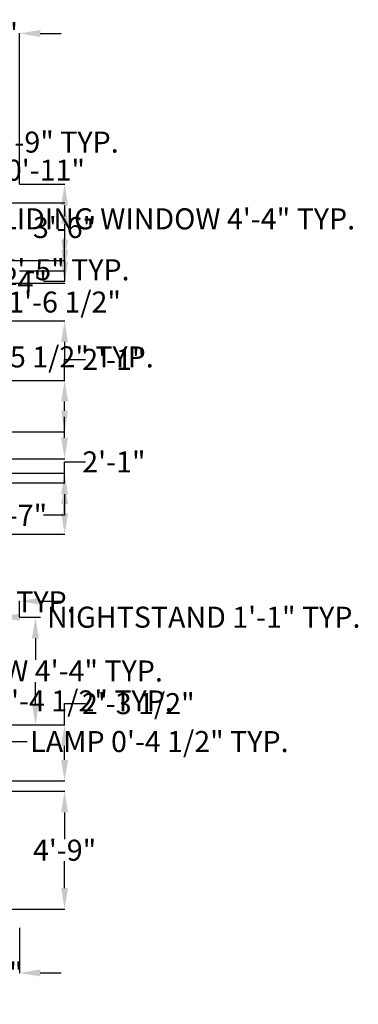
# Model space of a CAD drawing. Units: inches. Extents: x 19 to 1371, y 7 to 588.
# Tile 5 of 5: x 1207 to 1371, y 103 to 580. Entities that reach past the tile are written whole.
import ezdxf

# ---------------------------------------------------------------- set-up
doc = ezdxf.new("R2010")
doc.units = ezdxf.units.IN
doc.header["$MEASUREMENT"] = 0
doc.layers.add('A-ANNO-DIMS', color=2, linetype='Continuous', lineweight=18)
doc.styles.get("Standard").update_dxf_attribs({"font": 'arial.ttf'})
doc.dimstyles.get("Standard").update_dxf_attribs({"dimtxt": 10.18, "dimasz": 10.18, "dimexe": 0.18, "dimexo": 0.0625, "dimgap": 0.09, "dimtad": 0, "dimtih": 1, "dimtoh": 1, "dimdec": 0, "dimzin": 0, "dimdsep": 46, "dimlunit": 3, "dimtxsty": 'Standard', "dimcen": 0.09, "dimadec": 0, "dimazin": 0, "dimtfac": 1, "dimtdec": 0, "dimtofl": 0, "dimtmove": 0, "dimatfit": 3, "dimfxl": 1, "dimtolj": 1, "dimtzin": 0, "dimarcsym": 0})

# ---------------------------------------------------------------- blocks, each defined once
blk = doc.blocks.new('*D20')
at = {"layer": 'A-ANNO-DIMS', "color": 0, "lineweight": -2, "transparency": 16777216}
for p, q in [((1175.27, 490.89), (1185.12, 490.89)), ((1184.94, 480.71), (1184.94, 463.79)), ((1184.94, 436.16), (1184.94, 453.08)), ((1175.27, 425.98), (1185.12, 425.98))]:
    blk.add_line(p, q, dxfattribs=at)
at = {"layer": 'A-ANNO-DIMS', "color": 0, "transparency": 16777216}
for points in [[(1183.24, 480.71), (1186.64, 480.71), (1184.94, 490.89)], [(1183.24, 436.16), (1186.64, 436.16), (1184.94, 425.98)]]:
    blk.add_solid(points, dxfattribs=at)
at = {"layer": 'Defpoints', "color": 0, "transparency": 16777216}
for p in [(1175.2, 490.89), (1184.94, 490.89), (1175.2, 425.98)]:
    blk.add_point(p, dxfattribs=at)
at = {"layer": 'A-ANNO-DIMS', "color": 0, "transparency": 16777216, "insert": (1184.94, 458.44), "char_height": 10.18, "attachment_point": 5}
blk.add_mtext('\\A1;DOUBLE BED 5\'-5" TYP.', dxfattribs=at)
blk = doc.blocks.new('*D21')
at = {"layer": 'A-ANNO-DIMS', "color": 0, "lineweight": -2, "transparency": 16777216}
for p, q in [((1121.71, 425.92), (1121.71, 416.06)), ((1175.2, 425.92), (1175.2, 416.06)), ((1131.89, 416.24), (1165.02, 416.24)), ((1175.2, 416.24), (1185.38, 416.24))]:
    blk.add_line(p, q, dxfattribs=at)
at = {"layer": 'A-ANNO-DIMS', "color": 0, "transparency": 16777216}
for points in [[(1131.89, 417.94), (1131.89, 414.55), (1121.71, 416.24)], [(1165.02, 417.94), (1165.02, 414.55), (1175.2, 416.24)]]:
    blk.add_solid(points, dxfattribs=at)
at = {"layer": 'Defpoints', "color": 0, "transparency": 16777216}
for p in [(1121.71, 425.98), (1175.2, 425.98), (1175.2, 416.24)]:
    blk.add_point(p, dxfattribs=at)
at = {"layer": 'A-ANNO-DIMS', "color": 0, "transparency": 16777216, "insert": (1228.56, 416.24), "char_height": 10.18, "attachment_point": 5}
blk.add_mtext('\\A1;4\'-5 1/2" TYP.', dxfattribs=at)
blk = doc.blocks.new('*D22')
at = {"layer": 'A-ANNO-DIMS', "color": 0, "lineweight": -2, "transparency": 16777216}
for p, q in [((1183.48, 292.09), (1183.48, 290.03)), ((1196.42, 292.09), (1196.42, 290.03)), ((1173.3, 290.21), (1163.12, 290.21)), ((1206.6, 290.21), (1216.78, 290.21))]:
    blk.add_line(p, q, dxfattribs=at)
at = {"layer": 'A-ANNO-DIMS', "color": 0, "transparency": 16777216}
for points in [[(1173.3, 291.91), (1173.3, 288.52), (1183.48, 290.21)], [(1206.6, 291.91), (1206.6, 288.52), (1196.42, 290.21)]]:
    blk.add_solid(points, dxfattribs=at)
at = {"layer": 'Defpoints', "color": 0, "transparency": 16777216}
for p in [(1183.48, 292.15), (1196.42, 292.15), (1196.42, 290.21)]:
    blk.add_point(p, dxfattribs=at)
at = {"layer": 'A-ANNO-DIMS', "color": 0, "transparency": 16777216, "insert": (1295.84, 290.21), "char_height": 10.18, "attachment_point": 5}
blk.add_mtext('\\A1;NIGHTSTAND 1\'-1" TYP.', dxfattribs=at)
blk = doc.blocks.new('*D23')
at = {"layer": 'A-ANNO-DIMS', "color": 0, "lineweight": -2, "transparency": 16777216}
for p, q in [((1198.36, 313.34), (1198.36, 323.52)), ((1196.48, 303.16), (1198.54, 303.16)), ((1196.48, 292.15), (1198.54, 292.15)), ((1198.36, 281.97), (1198.36, 271.79))]:
    blk.add_line(p, q, dxfattribs=at)
at = {"layer": 'A-ANNO-DIMS', "color": 0, "transparency": 16777216}
for points in [[(1196.66, 313.34), (1200.05, 313.34), (1198.36, 303.16)], [(1196.66, 281.97), (1200.05, 281.97), (1198.36, 292.15)]]:
    blk.add_solid(points, dxfattribs=at)
at = {"layer": 'Defpoints', "color": 0, "transparency": 16777216}
for p in [(1196.42, 303.16), (1198.36, 303.16), (1196.42, 292.15)]:
    blk.add_point(p, dxfattribs=at)
at = {"layer": 'A-ANNO-DIMS', "color": 0, "transparency": 16777216, "insert": (1198.36, 297.66), "char_height": 10.18, "attachment_point": 5}
blk.add_mtext('\\A1;0\'-11" TYP.', dxfattribs=at)
blk = doc.blocks.new('*D24')
at = {"layer": 'A-ANNO-DIMS', "color": 0, "lineweight": -2, "transparency": 16777216}
for p, q in [((1175.14, 229.99), (1164.96, 229.99)), ((1185.32, 229.36), (1185.32, 230.17)), ((1189.92, 229.36), (1189.92, 230.17)), ((1200.1, 229.99), (1210.28, 229.99))]:
    blk.add_line(p, q, dxfattribs=at)
at = {"layer": 'A-ANNO-DIMS', "color": 0, "transparency": 16777216}
for points in [[(1175.14, 231.68), (1175.14, 228.29), (1185.32, 229.99)], [(1200.1, 231.68), (1200.1, 228.29), (1189.92, 229.99)]]:
    blk.add_solid(points, dxfattribs=at)
at = {"layer": 'Defpoints', "color": 0, "transparency": 16777216}
for p in [(1185.32, 229.3), (1189.92, 229.99), (1189.92, 229.3)]:
    blk.add_point(p, dxfattribs=at)
at = {"layer": 'A-ANNO-DIMS', "color": 0, "transparency": 16777216, "insert": (1274.37, 229.99), "char_height": 10.18, "attachment_point": 5}
blk.add_mtext('\\A1;LAMP 0\'-4 1/2" TYP.', dxfattribs=at)
blk = doc.blocks.new('*D25')
at = {"layer": 'A-ANNO-DIMS', "color": 0, "lineweight": -2, "transparency": 16777216}
for p, q in [((1184.63, 239.48), (1184.63, 249.66)), ((1184.63, 249.66), (1194.81, 249.66)), ((1185.26, 229.3), (1184.45, 229.3)), ((1185.26, 224.7), (1184.45, 224.7)), ((1184.63, 214.52), (1184.63, 204.34))]:
    blk.add_line(p, q, dxfattribs=at)
at = {"layer": 'A-ANNO-DIMS', "color": 0, "transparency": 16777216}
for points in [[(1182.93, 239.48), (1186.33, 239.48), (1184.63, 229.3)], [(1182.93, 214.52), (1186.33, 214.52), (1184.63, 224.7)]]:
    blk.add_solid(points, dxfattribs=at)
at = {"layer": 'Defpoints', "color": 0, "transparency": 16777216}
for p in [(1184.63, 229.3), (1185.32, 229.3), (1185.32, 224.7)]:
    blk.add_point(p, dxfattribs=at)
at = {"layer": 'A-ANNO-DIMS', "color": 0, "transparency": 16777216, "insert": (1237.79, 249.66), "char_height": 10.18, "attachment_point": 5}
blk.add_mtext('\\A1;0\'-4 1/2" TYP.', dxfattribs=at)
blk = doc.blocks.new('*D28')
at = {"layer": 'A-ANNO-DIMS', "color": 0, "lineweight": -2, "transparency": 16777216}
for p, q in [((1206.5, 290.16), (1214.42, 290.16)), ((1214.24, 279.98), (1214.24, 269.51)), ((1214.24, 248.34), (1214.24, 258.8)), ((1206.5, 238.16), (1214.42, 238.16))]:
    blk.add_line(p, q, dxfattribs=at)
at = {"layer": 'A-ANNO-DIMS', "color": 0, "transparency": 16777216}
for points in [[(1212.55, 279.98), (1215.94, 279.98), (1214.24, 290.16)], [(1212.55, 248.34), (1215.94, 248.34), (1214.24, 238.16)]]:
    blk.add_solid(points, dxfattribs=at)
at = {"layer": 'Defpoints', "color": 0, "transparency": 16777216}
for p in [(1206.44, 290.16), (1214.24, 290.16), (1206.44, 238.16)]:
    blk.add_point(p, dxfattribs=at)
at = {"layer": 'A-ANNO-DIMS', "color": 0, "transparency": 16777216, "insert": (1214.24, 264.16), "char_height": 10.18, "attachment_point": 5}
blk.add_mtext('\\A1;WINDOW 4\'-4" TYP.', dxfattribs=at)
blk = doc.blocks.new('*D29')
at = {"layer": 'A-ANNO-DIMS', "color": 0, "lineweight": -2, "transparency": 16777216}
for p, q in [((1187.26, 297.96), (1177.08, 297.96)), ((1197.44, 290.22), (1197.44, 298.14)), ((1206.44, 290.22), (1206.44, 298.14)), ((1216.62, 297.96), (1226.8, 297.96))]:
    blk.add_line(p, q, dxfattribs=at)
at = {"layer": 'A-ANNO-DIMS', "color": 0, "transparency": 16777216}
for points in [[(1187.26, 299.65), (1187.26, 296.26), (1197.44, 297.96)], [(1216.62, 299.65), (1216.62, 296.26), (1206.44, 297.96)]]:
    blk.add_solid(points, dxfattribs=at)
at = {"layer": 'Defpoints', "color": 0, "transparency": 16777216}
for p in [(1197.44, 297.96), (1197.44, 290.16), (1206.44, 290.16)]:
    blk.add_point(p, dxfattribs=at)
at = {"layer": 'A-ANNO-DIMS', "color": 0, "transparency": 16777216, "insert": (1145.97, 297.96), "char_height": 10.18, "attachment_point": 5}
blk.add_mtext('\\A1;0\'-9" TYP.', dxfattribs=at)
blk = doc.blocks.new('*D30')
at = {"layer": 'A-ANNO-DIMS', "color": 0, "lineweight": -2, "transparency": 16777216}
for p, q in [((1122.46, 490.83), (1122.46, 482.91)), ((1174.46, 490.83), (1174.46, 482.91)), ((1132.64, 483.09), (1164.28, 483.09)), ((1174.46, 483.09), (1184.64, 483.09))]:
    blk.add_line(p, q, dxfattribs=at)
at = {"layer": 'A-ANNO-DIMS', "color": 0, "transparency": 16777216}
for points in [[(1132.64, 484.79), (1132.64, 481.39), (1122.46, 483.09)], [(1164.28, 484.79), (1164.28, 481.39), (1174.46, 483.09)]]:
    blk.add_solid(points, dxfattribs=at)
at = {"layer": 'Defpoints', "color": 0, "transparency": 16777216}
for p in [(1122.46, 490.89), (1174.46, 490.89), (1174.46, 483.09)]:
    blk.add_point(p, dxfattribs=at)
at = {"layer": 'A-ANNO-DIMS', "color": 0, "transparency": 16777216, "insert": (1279.33, 483.09), "char_height": 10.18, "attachment_point": 5}
blk.add_mtext('\\A1;SLIDING WINDOW 4\'-4" TYP.', dxfattribs=at)
blk = doc.blocks.new('*D31')
at = {"layer": 'A-ANNO-DIMS', "color": 0, "lineweight": -2, "transparency": 16777216}
for p, q in [((1182.26, 510.07), (1182.26, 520.25)), ((1182.26, 520.25), (1192.44, 520.25)), ((1174.52, 499.89), (1182.44, 499.89)), ((1174.52, 490.89), (1182.44, 490.89)), ((1182.26, 480.71), (1182.26, 470.53))]:
    blk.add_line(p, q, dxfattribs=at)
at = {"layer": 'A-ANNO-DIMS', "color": 0, "transparency": 16777216}
for points in [[(1180.56, 510.07), (1183.95, 510.07), (1182.26, 499.89)], [(1180.56, 480.71), (1183.95, 480.71), (1182.26, 490.89)]]:
    blk.add_solid(points, dxfattribs=at)
at = {"layer": 'Defpoints', "color": 0, "transparency": 16777216}
for p in [(1174.46, 499.89), (1182.26, 499.89), (1174.46, 490.89)]:
    blk.add_point(p, dxfattribs=at)
at = {"layer": 'A-ANNO-DIMS', "color": 0, "transparency": 16777216, "insert": (1223.55, 520.25), "char_height": 10.18, "attachment_point": 5}
blk.add_mtext('\\A1;0\'-9" TYP.', dxfattribs=at)
blk = doc.blocks.new('*D48')
at = {"layer": 'A-ANNO-DIMS', "color": 0, "lineweight": -2, "transparency": 16777216}
for p, q in [((1228.39, 404.87), (1228.39, 415.05)), ((1228.39, 415.05), (1238.57, 415.05)), ((1093.5, 404.87), (1228.57, 404.87)), ((1228.39, 390.2), (1228.39, 394.69)), ((1093.23, 380.02), (1228.57, 380.02))]:
    blk.add_line(p, q, dxfattribs=at)
at = {"layer": 'A-ANNO-DIMS', "color": 0, "transparency": 16777216}
for points in [[(1226.7, 394.69), (1230.09, 394.69), (1228.39, 404.87)], [(1226.7, 390.2), (1230.09, 390.2), (1228.39, 380.02)]]:
    blk.add_solid(points, dxfattribs=at)
at = {"layer": 'Defpoints', "color": 0, "transparency": 16777216}
for p in [(1093.44, 404.87), (1228.39, 404.87), (1093.17, 380.02)]:
    blk.add_point(p, dxfattribs=at)
at = {"layer": 'A-ANNO-DIMS', "color": 0, "transparency": 16777216, "insert": (1252.28, 415.05), "char_height": 10.18, "attachment_point": 5}
blk.add_mtext('\\A1;2\'-1"', dxfattribs=at)
blk = doc.blocks.new('*D49')
at = {"layer": 'A-ANNO-DIMS', "color": 0, "lineweight": -2, "transparency": 16777216}
for p, q in [((1228.39, 355.24), (1228.39, 365.42)), ((1228.39, 365.42), (1238.57, 365.42)), ((1093.5, 355.24), (1228.57, 355.24)), ((1228.39, 340.57), (1228.39, 345.06)), ((1093.5, 330.39), (1228.57, 330.39))]:
    blk.add_line(p, q, dxfattribs=at)
at = {"layer": 'A-ANNO-DIMS', "color": 0, "transparency": 16777216}
for points in [[(1226.7, 345.06), (1230.09, 345.06), (1228.39, 355.24)], [(1226.7, 340.57), (1230.09, 340.57), (1228.39, 330.39)]]:
    blk.add_solid(points, dxfattribs=at)
at = {"layer": 'Defpoints', "color": 0, "transparency": 16777216}
for p in [(1093.44, 355.24), (1228.39, 355.24), (1093.44, 330.39)]:
    blk.add_point(p, dxfattribs=at)
at = {"layer": 'A-ANNO-DIMS', "color": 0, "transparency": 16777216, "insert": (1252.28, 365.42), "char_height": 10.18, "attachment_point": 5}
blk.add_mtext('\\A1;2\'-1"', dxfattribs=at)
blk = doc.blocks.new('*D50')
at = {"layer": 'A-ANNO-DIMS', "color": 0, "lineweight": -2, "transparency": 16777216}
for p, q in [((1228.39, 462.14), (1228.39, 472.32)), ((1093.5, 451.96), (1228.57, 451.96)), ((1093.5, 433.64), (1228.57, 433.64)), ((1228.39, 423.46), (1228.39, 413.28))]:
    blk.add_line(p, q, dxfattribs=at)
at = {"layer": 'A-ANNO-DIMS', "color": 0, "transparency": 16777216}
for points in [[(1226.7, 462.14), (1230.09, 462.14), (1228.39, 451.96)], [(1226.7, 423.46), (1230.09, 423.46), (1228.39, 433.64)]]:
    blk.add_solid(points, dxfattribs=at)
at = {"layer": 'Defpoints', "color": 0, "transparency": 16777216}
for p in [(1093.44, 451.96), (1228.39, 451.96), (1093.44, 433.64)]:
    blk.add_point(p, dxfattribs=at)
at = {"layer": 'A-ANNO-DIMS', "color": 0, "transparency": 16777216, "insert": (1228.39, 442.8), "char_height": 10.18, "attachment_point": 5}
blk.add_mtext('\\A1;1\'-6 1/2"', dxfattribs=at)
blk = doc.blocks.new('*D54')
at = {"layer": 'A-ANNO-DIMS', "color": 0, "lineweight": -2, "transparency": 16777216}
for p, q in [((1197.5, 205.89), (1228.57, 205.89)), ((1228.39, 195.71), (1228.39, 182.68)), ((1228.39, 159.07), (1228.39, 172.1)), ((1197.5, 148.89), (1228.57, 148.89))]:
    blk.add_line(p, q, dxfattribs=at)
at = {"layer": 'A-ANNO-DIMS', "color": 0, "transparency": 16777216}
for points in [[(1226.7, 195.71), (1230.09, 195.71), (1228.39, 205.89)], [(1226.7, 159.07), (1230.09, 159.07), (1228.39, 148.89)]]:
    blk.add_solid(points, dxfattribs=at)
at = {"layer": 'Defpoints', "color": 0, "transparency": 16777216}
for p in [(1197.44, 205.89), (1228.39, 205.89), (1197.44, 148.89)]:
    blk.add_point(p, dxfattribs=at)
at = {"layer": 'A-ANNO-DIMS', "color": 0, "transparency": 16777216, "insert": (1228.39, 177.39), "char_height": 10.18, "attachment_point": 5}
blk.add_mtext('\\A1;4\'-9"', dxfattribs=at)
blk = doc.blocks.new('*D61')
at = {"layer": 'A-ANNO-DIMS', "color": 0, "lineweight": -2, "transparency": 16777216}
for p, q in [((1206.5, 499.89), (1228.57, 499.89)), ((1228.39, 489.71), (1228.39, 484.18)), ((1228.39, 468.07), (1228.39, 473.6)), ((1206.5, 457.89), (1228.57, 457.89))]:
    blk.add_line(p, q, dxfattribs=at)
at = {"layer": 'A-ANNO-DIMS', "color": 0, "transparency": 16777216}
for points in [[(1226.7, 489.71), (1230.09, 489.71), (1228.39, 499.89)], [(1226.7, 468.07), (1230.09, 468.07), (1228.39, 457.89)]]:
    blk.add_solid(points, dxfattribs=at)
at = {"layer": 'Defpoints', "color": 0, "transparency": 16777216}
for p in [(1206.44, 499.89), (1206.44, 457.89), (1228.39, 457.89)]:
    blk.add_point(p, dxfattribs=at)
at = {"layer": 'A-ANNO-DIMS', "color": 0, "transparency": 16777216, "insert": (1228.39, 478.89), "char_height": 10.18, "attachment_point": 5}
blk.add_mtext('\\A1;3\'-6"', dxfattribs=at)
blk = doc.blocks.new('*D62')
at = {"layer": 'A-ANNO-DIMS', "color": 0, "lineweight": -2, "transparency": 16777216}
for p, q in [((1228.39, 377.07), (1228.39, 387.25)), ((1197.5, 366.89), (1228.57, 366.89)), ((1197.5, 359.89), (1228.57, 359.89)), ((1228.39, 349.71), (1228.39, 339.53)), ((1228.39, 339.53), (1218.21, 339.53))]:
    blk.add_line(p, q, dxfattribs=at)
at = {"layer": 'A-ANNO-DIMS', "color": 0, "transparency": 16777216}
for points in [[(1226.7, 377.07), (1230.09, 377.07), (1228.39, 366.89)], [(1226.7, 349.71), (1230.09, 349.71), (1228.39, 359.89)]]:
    blk.add_solid(points, dxfattribs=at)
at = {"layer": 'Defpoints', "color": 0, "transparency": 16777216}
for p in [(1197.44, 366.89), (1197.44, 359.89), (1228.39, 359.89)]:
    blk.add_point(p, dxfattribs=at)
at = {"layer": 'A-ANNO-DIMS', "color": 0, "transparency": 16777216, "insert": (1204.59, 339.53), "char_height": 10.18, "attachment_point": 5}
blk.add_mtext('\\A1;0\'-7"', dxfattribs=at)
blk = doc.blocks.new('*D63')
at = {"layer": 'A-ANNO-DIMS', "color": 0, "lineweight": -2, "transparency": 16777216}
for p, q in [((1228.39, 238.16), (1228.39, 248.34)), ((1228.39, 248.34), (1238.57, 248.34)), ((1197.5, 238.16), (1228.57, 238.16)), ((1228.39, 221.07), (1228.39, 227.98)), ((1197.5, 210.89), (1228.57, 210.89))]:
    blk.add_line(p, q, dxfattribs=at)
at = {"layer": 'A-ANNO-DIMS', "color": 0, "transparency": 16777216}
for points in [[(1226.7, 227.98), (1230.09, 227.98), (1228.39, 238.16)], [(1226.7, 221.07), (1230.09, 221.07), (1228.39, 210.89)]]:
    blk.add_solid(points, dxfattribs=at)
at = {"layer": 'Defpoints', "color": 0, "transparency": 16777216}
for p in [(1197.44, 238.16), (1228.39, 238.16), (1197.44, 210.89)]:
    blk.add_point(p, dxfattribs=at)
at = {"layer": 'A-ANNO-DIMS', "color": 0, "transparency": 16777216, "insert": (1264.14, 248.34), "char_height": 10.18, "attachment_point": 5}
blk.add_mtext('\\A1;2\'-3 1/2"', dxfattribs=at)
blk = doc.blocks.new('*D65')
at = {"layer": 'A-ANNO-DIMS', "color": 0, "lineweight": -2, "transparency": 16777216}
for p, q in [((1164.28, 572.84), (1154.1, 572.84)), ((1174.46, 499.95), (1174.46, 573.02)), ((1206.44, 499.95), (1206.44, 573.02)), ((1216.62, 572.84), (1226.8, 572.84))]:
    blk.add_line(p, q, dxfattribs=at)
at = {"layer": 'A-ANNO-DIMS', "color": 0, "transparency": 16777216}
for points in [[(1164.28, 574.54), (1164.28, 571.14), (1174.46, 572.84)], [(1216.62, 574.54), (1216.62, 571.14), (1206.44, 572.84)]]:
    blk.add_solid(points, dxfattribs=at)
at = {"layer": 'Defpoints', "color": 0, "transparency": 16777216}
for p in [(1206.44, 572.84), (1174.46, 499.89), (1206.44, 499.89)]:
    blk.add_point(p, dxfattribs=at)
at = {"layer": 'A-ANNO-DIMS', "color": 0, "transparency": 16777216, "insert": (1190.45, 572.84), "char_height": 10.18, "attachment_point": 5}
blk.add_mtext('\\A1;2\'-8"', dxfattribs=at)
blk = doc.blocks.new('*D67')
at = {"layer": 'A-ANNO-DIMS', "color": 0, "lineweight": -2, "transparency": 16777216}
for p, q in [((1154.94, 139.83), (1154.94, 117.76)), ((1206.44, 139.83), (1206.44, 117.76)), ((1144.76, 117.94), (1134.58, 117.94)), ((1216.62, 117.94), (1226.8, 117.94))]:
    blk.add_line(p, q, dxfattribs=at)
at = {"layer": 'A-ANNO-DIMS', "color": 0, "transparency": 16777216}
for points in [[(1144.76, 119.64), (1144.76, 116.24), (1154.94, 117.94)], [(1216.62, 119.64), (1216.62, 116.24), (1206.44, 117.94)]]:
    blk.add_solid(points, dxfattribs=at)
at = {"layer": 'Defpoints', "color": 0, "transparency": 16777216}
for p in [(1154.94, 139.89), (1206.44, 139.89), (1206.44, 117.94)]:
    blk.add_point(p, dxfattribs=at)
at = {"layer": 'A-ANNO-DIMS', "color": 0, "transparency": 16777216, "insert": (1180.69, 117.94), "char_height": 10.18, "attachment_point": 5}
blk.add_mtext('\\A1;4\'-3 1/2"', dxfattribs=at)
blk = doc.blocks.new('*D69')
at = {"layer": 'A-ANNO-DIMS', "color": 0, "lineweight": -2, "transparency": 16777216}
for p, q in [((1080.93, 490.89), (1228.57, 490.89)), ((1228.39, 480.71), (1228.39, 473.07)), ((1070.43, 462.89), (1228.57, 462.89)), ((1228.39, 462.89), (1228.39, 452.71)), ((1228.39, 452.71), (1218.21, 452.71))]:
    blk.add_line(p, q, dxfattribs=at)
at = {"layer": 'A-ANNO-DIMS', "color": 0, "transparency": 16777216}
for points in [[(1226.7, 480.71), (1230.09, 480.71), (1228.39, 490.89)], [(1226.7, 473.07), (1230.09, 473.07), (1228.39, 462.89)]]:
    blk.add_solid(points, dxfattribs=at)
at = {"layer": 'Defpoints', "color": 0, "transparency": 16777216}
for p in [(1080.87, 490.89), (1070.37, 462.89), (1228.39, 462.89)]:
    blk.add_point(p, dxfattribs=at)
at = {"layer": 'A-ANNO-DIMS', "color": 0, "transparency": 16777216, "insert": (1204.51, 452.71), "char_height": 10.18, "attachment_point": 5}
blk.add_mtext('\\A1;2\'-4"', dxfattribs=at)
blk = doc.blocks.new('*D75')
at = {"layer": 'A-ANNO-DIMS', "color": 0, "lineweight": -2, "transparency": 16777216}
for p, q in [((1171.71, 506.67), (1161.53, 506.67)), ((1161.53, 506.67), (1161.53, 496.49)), ((1161.44, 475.42), (1161.62, 475.42)), ((1161.53, 475.33), (1161.53, 475.51))]:
    blk.add_line(p, q, dxfattribs=at)
at = {"layer": 'A-ANNO-DIMS', "color": 0, "transparency": 16777216}
blk.add_solid([(1159.84, 496.49), (1163.23, 496.49), (1161.53, 486.31)], dxfattribs=at)
at = {"layer": 'Defpoints', "color": 0, "transparency": 16777216}
for p in [(1161.53, 486.31), (1161.53, 475.42)]:
    blk.add_point(p, dxfattribs=at)
at = {"layer": 'A-ANNO-DIMS', "color": 0, "transparency": 16777216, "insert": (1205.3, 506.67), "char_height": 10.18, "attachment_point": 5}
blk.add_mtext('\\A1;4X R0\'-11"', dxfattribs=at)

msp = doc.modelspace()

# ---------------------------------------------------------------- dimensions: what is measured, and where the dimension line sits
at = {"layer": 'A-ANNO-DIMS'}
for base, p1, p2, picture, middle in [((1206.44, 572.84), (1174.46, 499.89), (1206.44, 499.89), '*D65', (1190.45, 572.84)), ((1206.44, 117.94), (1154.94, 139.89), (1206.44, 139.89), '*D67', (1180.69, 117.94))]:
    dim = msp.add_linear_dim(base=base, p1=p1, p2=p2, dimstyle='Standard', override={"dimdec": 1, "dimlfac": 1, "dimrnd": 0, "dimzin": 1, "dimdsep": 46, "dimlunit": 4, "dimfrac": 2}, dxfattribs=at)
    dim.commit()
    dim.dimension.update_dxf_attribs({"geometry": picture, "text_midpoint": middle})
for base, p1, p2, angle, text, picture, middle in [((1182.26, 499.89), (1174.46, 490.89), (1174.46, 499.89), 90, '<> TYP.', '*D31', (1223.55, 520.25)), ((1184.94, 490.89), (1175.2, 425.98), (1175.2, 490.89), 90, 'DOUBLE BED <> TYP.', '*D20', (1184.94, 458.44)), ((1198.36, 303.16), (1196.42, 292.15), (1196.42, 303.16), 90, '<> TYP.', '*D23', (1198.36, 297.66)), ((1197.44, 297.96), (1206.44, 290.16), (1197.44, 290.16), 180, '<> TYP.', '*D29', (1145.97, 297.96)), ((1214.24, 290.16), (1206.44, 238.16), (1206.44, 290.16), 90, 'WINDOW <> TYP.', '*D28', (1214.24, 264.16)), ((1184.63, 229.3), (1185.32, 224.7), (1185.32, 229.3), 90, '<> TYP.', '*D25', (1237.79, 249.66))]:
    dim = msp.add_linear_dim(base=base, p1=p1, p2=p2, angle=angle, text=text, dimstyle='Standard', override={"dimdec": 1, "dimlfac": 1, "dimrnd": 0, "dimzin": 1, "dimdsep": 46, "dimlunit": 4, "dimfrac": 2}, dxfattribs=at)
    dim.commit()
    dim.dimension.update_dxf_attribs({"geometry": picture, "text_midpoint": middle})
dim = msp.add_radius_dim(center=(1161.53, 475.42), mpoint=(1161.53, 486.31), text='4X <>', dimstyle='Standard', override={"dimdec": 1, "dimlfac": 1, "dimrnd": 0, "dimzin": 1, "dimdsep": 46, "dimlunit": 4, "dimfrac": 2}, dxfattribs=at)
dim.commit()
dim.dimension.update_dxf_attribs({"geometry": '*D75', "text_midpoint": (1205.3, 506.67)})
for base, p1, p2, text, picture, middle in [((1174.46, 483.09), (1122.46, 490.89), (1174.46, 490.89), 'SLIDING WINDOW <> TYP.', '*D30', (1279.33, 483.09)), ((1175.2, 416.24), (1121.71, 425.98), (1175.2, 425.98), '<> TYP.', '*D21', (1228.56, 416.24)), ((1196.42, 290.21), (1183.48, 292.15), (1196.42, 292.15), 'NIGHTSTAND <> TYP.', '*D22', (1295.84, 290.21)), ((1189.92, 229.99), (1185.32, 229.3), (1189.92, 229.3), 'LAMP <> TYP.', '*D24', (1274.37, 229.99))]:
    dim = msp.add_linear_dim(base=base, p1=p1, p2=p2, text=text, dimstyle='Standard', override={"dimdec": 1, "dimlfac": 1, "dimrnd": 0, "dimzin": 1, "dimdsep": 46, "dimlunit": 4, "dimfrac": 2}, dxfattribs=at)
    dim.commit()
    dim.dimension.update_dxf_attribs({"geometry": picture, "text_midpoint": middle})
for base, p1, p2, picture, middle in [((1228.39, 457.89), (1206.44, 499.89), (1206.44, 457.89), '*D61', (1228.39, 478.89)), ((1228.39, 462.89), (1080.87, 490.89), (1070.37, 462.89), '*D69', (1204.51, 452.71)), ((1228.39, 451.96), (1093.44, 433.64), (1093.44, 451.96), '*D50', (1228.39, 442.8)), ((1228.39246, 404.87298), (1093.17018, 380.02295), (1093.44246, 404.87298), '*D48', (1252.27977, 415.05298)), ((1228.39, 359.89), (1197.44, 366.89), (1197.44, 359.89), '*D62', (1204.59, 339.53)), ((1228.39246, 355.24399), (1093.44246, 330.39396), (1093.44246, 355.24399), '*D49', (1252.27977, 365.42399)), ((1228.39, 238.16), (1197.44, 210.89), (1197.44, 238.16), '*D63', (1264.14, 248.34)), ((1228.39, 205.89), (1197.44, 148.89), (1197.44, 205.89), '*D54', (1228.39, 177.39))]:
    dim = msp.add_linear_dim(base=base, p1=p1, p2=p2, angle=90, dimstyle='Standard', override={"dimdec": 1, "dimlfac": 1, "dimrnd": 0, "dimzin": 1, "dimdsep": 46, "dimlunit": 4, "dimfrac": 2}, dxfattribs=at)
    dim.commit()
    dim.dimension.update_dxf_attribs({"geometry": picture, "text_midpoint": middle})

doc.saveas('drawing.dxf')
